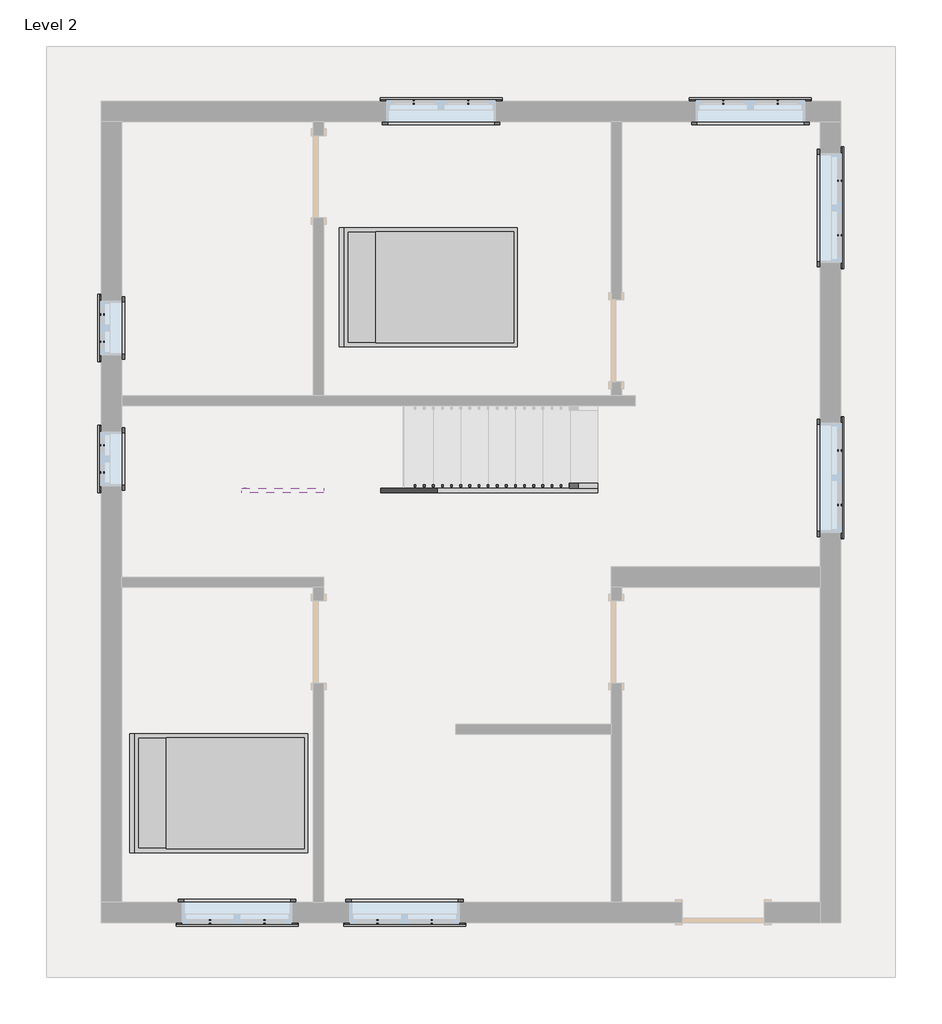
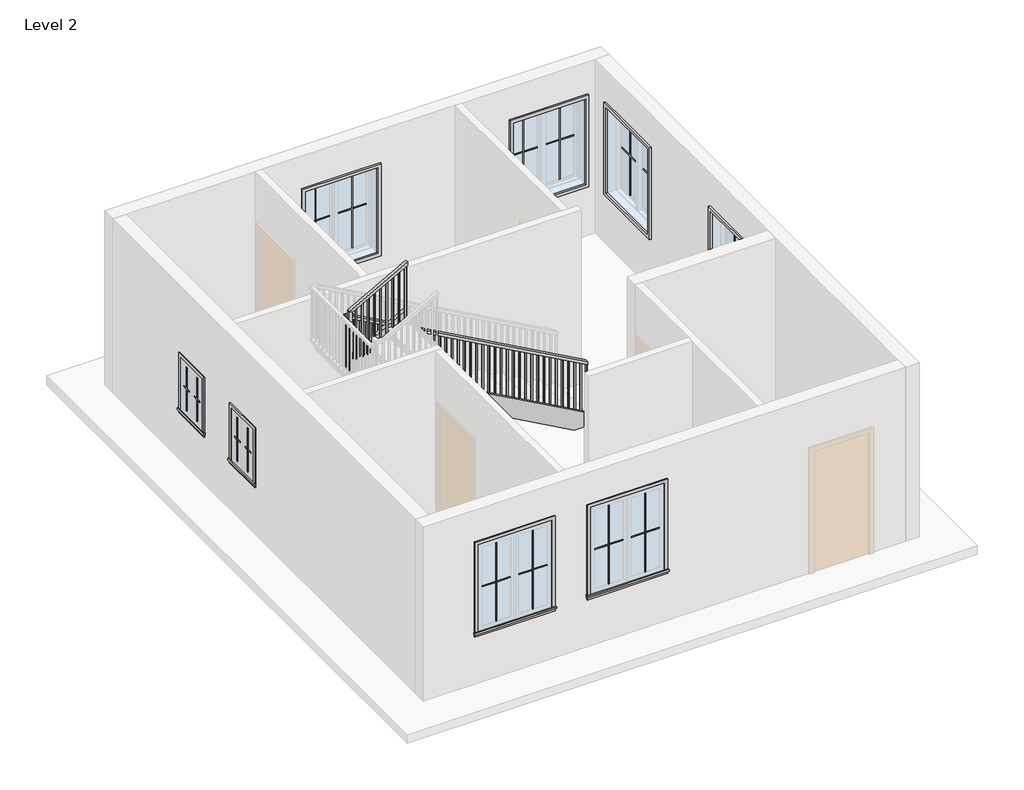
# One storey, part 2 of 2: 32 proxies, 3 members, 2 furniture elements, 1 railing.
"""IFC4 building model written with IfcOpenShell, lengths in millimetres."""

from ifc_helpers import new_model, si_unit, frame, origin, place, context, project, spatial, polyline, outline, extrude, faceted_brep, transform, mapped, element, save
from components import muntin_pattern_2x2_muntin_pattern_2x2_53152e2c, muntin_pattern_2x2_muntin_pattern_2x2_e8f3e573, muntin_pattern_2x2_muntin_pattern_2x2_6dad3731, muntin_pattern_2x2_muntin_pattern_2x2_a30a3345, trim_window_exterior_flat_with_sill_a665a915, trim_window_exterior_flat_with_sill_92b9b949, trim_window_interior_flat_picture_frame_d485c387, trim_window_interior_flat_picture_frame_3bb882cf, bed_17739_bed_17739_15c61121

model = new_model("IFC4")

# Units and contexts
model_context = context("Model", 3, world=origin())
ifc_project = project(units=[si_unit("LENGTHUNIT", "METRE", prefix="MILLI")], contexts=[model_context])

# Site, building, storey
site = spatial("IfcSite", under=ifc_project)
building = spatial("IfcBuilding", under=site)
storey = spatial("IfcBuildingStorey", under=building, Name="Level 2", Elevation=3048.0)

# Proxies
placement = place(None, origin())
muntin_pattern_2x2_muntin_pattern_2x2_shape = muntin_pattern_2x2_muntin_pattern_2x2_53152e2c(model_context)
element("IfcBuildingElementProxy", 1, Name="Muntin Pattern_2x2 : Muntin Pattern_2x2", ObjectType="Muntin Pattern_2x2 : Muntin Pattern_2x2", at=placement, inside=storey, context=model_context, shape_type="MappedRepresentation", body=[
    mapped(muntin_pattern_2x2_muntin_pattern_2x2_shape, transform((1279.525, 12101.9997886, 4032.25), x_axis=(0.0, 1.0, 0.0), y_axis=(-1.0, 0.0, 0.0), z_axis=(0.0, 0.0, 1.0))),
])
element("IfcBuildingElementProxy", 2, Name="Muntin Pattern_2x2 : Muntin Pattern_2x2", ObjectType="Muntin Pattern_2x2 : Muntin Pattern_2x2", at=placement, inside=storey, context=model_context, shape_type="MappedRepresentation", body=[
    mapped(muntin_pattern_2x2_muntin_pattern_2x2_shape, transform((1279.525, 10644.6747886, 4032.25), x_axis=(0.0, 1.0, 0.0), y_axis=(-1.0, 0.0, 0.0), z_axis=(0.0, 0.0, 1.0))),
])
muntin_pattern_2x2_muntin_pattern_2x2_2_shape = muntin_pattern_2x2_muntin_pattern_2x2_e8f3e573(model_context)
element("IfcBuildingElementProxy", 3, Name="Muntin Pattern_2x2 : Muntin Pattern_2x2", ObjectType="Muntin Pattern_2x2 : Muntin Pattern_2x2", at=placement, inside=storey, context=model_context, shape_type="MappedRepresentation", body=[
    mapped(muntin_pattern_2x2_muntin_pattern_2x2_2_shape, transform((1279.525, 12403.6247886, 4032.25), x_axis=(0.0, -1.0, 0.0), y_axis=(1.0, 0.0, 0.0), z_axis=(0.0, 0.0, 1.0))),
])
element("IfcBuildingElementProxy", 4, Name="Muntin Pattern_2x2 : Muntin Pattern_2x2", ObjectType="Muntin Pattern_2x2 : Muntin Pattern_2x2", at=placement, inside=storey, context=model_context, shape_type="MappedRepresentation", body=[
    mapped(muntin_pattern_2x2_muntin_pattern_2x2_2_shape, transform((1279.525, 10946.2997886, 4032.25), x_axis=(0.0, -1.0, 0.0), y_axis=(1.0, 0.0, 0.0), z_axis=(0.0, 0.0, 1.0))),
])
muntin_pattern_2x2_muntin_pattern_2x2_3_shape = muntin_pattern_2x2_muntin_pattern_2x2_6dad3731(model_context)
element("IfcBuildingElementProxy", 5, Name="Muntin Pattern_2x2 : Muntin Pattern_2x2", ObjectType="Muntin Pattern_2x2 : Muntin Pattern_2x2", at=placement, inside=storey, context=model_context, shape_type="MappedRepresentation", body=[
    mapped(muntin_pattern_2x2_muntin_pattern_2x2_3_shape, transform((9490.075, 13892.6997886, 4032.25), x_axis=(0.0, -1.0, 0.0), y_axis=(1.0, 0.0, 0.0), z_axis=(0.0, 0.0, 1.0))),
])
element("IfcBuildingElementProxy", 6, Name="Muntin Pattern_2x2 : Muntin Pattern_2x2", ObjectType="Muntin Pattern_2x2 : Muntin Pattern_2x2", at=placement, inside=storey, context=model_context, shape_type="MappedRepresentation", body=[
    mapped(muntin_pattern_2x2_muntin_pattern_2x2_3_shape, transform((8193.0875, 14767.4122886, 4032.25), x_axis=(1.0, 0.0, 0.0), y_axis=(0.0, 1.0, 0.0), z_axis=(0.0, 0.0, 1.0))),
])
element("IfcBuildingElementProxy", 7, Name="Muntin Pattern_2x2 : Muntin Pattern_2x2", ObjectType="Muntin Pattern_2x2 : Muntin Pattern_2x2", at=placement, inside=storey, context=model_context, shape_type="MappedRepresentation", body=[
    mapped(muntin_pattern_2x2_muntin_pattern_2x2_3_shape, transform((4749.8, 14767.4122886, 4032.25), x_axis=(1.0, 0.0, 0.0), y_axis=(0.0, 1.0, 0.0), z_axis=(0.0, 0.0, 1.0))),
])
element("IfcBuildingElementProxy", 8, Name="Muntin Pattern_2x2 : Muntin Pattern_2x2", ObjectType="Muntin Pattern_2x2 : Muntin Pattern_2x2", at=placement, inside=storey, context=model_context, shape_type="MappedRepresentation", body=[
    mapped(muntin_pattern_2x2_muntin_pattern_2x2_3_shape, transform((9490.075, 10889.1497886, 4032.25), x_axis=(0.0, -1.0, 0.0), y_axis=(1.0, 0.0, 0.0), z_axis=(0.0, 0.0, 1.0))),
])
element("IfcBuildingElementProxy", 9, Name="Muntin Pattern_2x2 : Muntin Pattern_2x2", ObjectType="Muntin Pattern_2x2 : Muntin Pattern_2x2", at=placement, inside=storey, context=model_context, shape_type="MappedRepresentation", body=[
    mapped(muntin_pattern_2x2_muntin_pattern_2x2_3_shape, transform((4950.6207347, 5642.4622886, 4032.25), x_axis=(-1.0, 0.0, 0.0), y_axis=(0.0, -1.0, 0.0), z_axis=(0.0, 0.0, 1.0))),
])
element("IfcBuildingElementProxy", 10, Name="Muntin Pattern_2x2 : Muntin Pattern_2x2", ObjectType="Muntin Pattern_2x2 : Muntin Pattern_2x2", at=placement, inside=storey, context=model_context, shape_type="MappedRepresentation", body=[
    mapped(muntin_pattern_2x2_muntin_pattern_2x2_3_shape, transform((3086.1019847, 5642.4622886, 4032.25), x_axis=(-1.0, 0.0, 0.0), y_axis=(0.0, -1.0, 0.0), z_axis=(0.0, 0.0, 1.0))),
])
muntin_pattern_2x2_muntin_pattern_2x2_4_shape = muntin_pattern_2x2_muntin_pattern_2x2_a30a3345(model_context)
element("IfcBuildingElementProxy", 11, Name="Muntin Pattern_2x2 : Muntin Pattern_2x2", ObjectType="Muntin Pattern_2x2 : Muntin Pattern_2x2", at=placement, inside=storey, context=model_context, shape_type="MappedRepresentation", body=[
    mapped(muntin_pattern_2x2_muntin_pattern_2x2_4_shape, transform((9490.075, 13286.2747886, 4032.25), x_axis=(0.0, 1.0, 0.0), y_axis=(-1.0, 0.0, 0.0), z_axis=(0.0, 0.0, 1.0))),
])
element("IfcBuildingElementProxy", 12, Name="Muntin Pattern_2x2 : Muntin Pattern_2x2", ObjectType="Muntin Pattern_2x2 : Muntin Pattern_2x2", at=placement, inside=storey, context=model_context, shape_type="MappedRepresentation", body=[
    mapped(muntin_pattern_2x2_muntin_pattern_2x2_4_shape, transform((8799.5125, 14767.4122886, 4032.25), x_axis=(-1.0, 0.0, 0.0), y_axis=(0.0, -1.0, 0.0), z_axis=(0.0, 0.0, 1.0))),
])
element("IfcBuildingElementProxy", 13, Name="Muntin Pattern_2x2 : Muntin Pattern_2x2", ObjectType="Muntin Pattern_2x2 : Muntin Pattern_2x2", at=placement, inside=storey, context=model_context, shape_type="MappedRepresentation", body=[
    mapped(muntin_pattern_2x2_muntin_pattern_2x2_4_shape, transform((5356.225, 14767.4122886, 4032.25), x_axis=(-1.0, 0.0, 0.0), y_axis=(0.0, -1.0, 0.0), z_axis=(0.0, 0.0, 1.0))),
])
element("IfcBuildingElementProxy", 14, Name="Muntin Pattern_2x2 : Muntin Pattern_2x2", ObjectType="Muntin Pattern_2x2 : Muntin Pattern_2x2", at=placement, inside=storey, context=model_context, shape_type="MappedRepresentation", body=[
    mapped(muntin_pattern_2x2_muntin_pattern_2x2_4_shape, transform((9490.075, 10282.7247886, 4032.25), x_axis=(0.0, 1.0, 0.0), y_axis=(-1.0, 0.0, 0.0), z_axis=(0.0, 0.0, 1.0))),
])
element("IfcBuildingElementProxy", 15, Name="Muntin Pattern_2x2 : Muntin Pattern_2x2", ObjectType="Muntin Pattern_2x2 : Muntin Pattern_2x2", at=placement, inside=storey, context=model_context, shape_type="MappedRepresentation", body=[
    mapped(muntin_pattern_2x2_muntin_pattern_2x2_4_shape, transform((4344.1957347, 5642.4622886, 4032.25), x_axis=(1.0, 0.0, 0.0), y_axis=(0.0, 1.0, 0.0), z_axis=(0.0, 0.0, 1.0))),
])
element("IfcBuildingElementProxy", 16, Name="Muntin Pattern_2x2 : Muntin Pattern_2x2", ObjectType="Muntin Pattern_2x2 : Muntin Pattern_2x2", at=placement, inside=storey, context=model_context, shape_type="MappedRepresentation", body=[
    mapped(muntin_pattern_2x2_muntin_pattern_2x2_4_shape, transform((2479.6769847, 5642.4622886, 4032.25), x_axis=(1.0, 0.0, 0.0), y_axis=(0.0, 1.0, 0.0), z_axis=(0.0, 0.0, 1.0))),
])
trim_window_exterior_flat_with_sill_shape = trim_window_exterior_flat_with_sill_a665a915(model_context)
element("IfcBuildingElementProxy", 17, Name="Trim-Window-Exterior-Flat : with Sill", ObjectType="Trim-Window-Exterior-Flat : with Sill", at=placement, inside=storey, context=model_context, shape_type="MappedRepresentation", body=[
    mapped(trim_window_exterior_flat_with_sill_shape, transform((1270.0, 12252.8122886, 4876.8), x_axis=(0.0, -1.0, 0.0), y_axis=(0.0, 0.0, 1.0), z_axis=(-1.0, 0.0, 0.0))),
])
element("IfcBuildingElementProxy", 18, Name="Trim-Window-Exterior-Flat : with Sill", ObjectType="Trim-Window-Exterior-Flat : with Sill", at=placement, inside=storey, context=model_context, shape_type="MappedRepresentation", body=[
    mapped(trim_window_exterior_flat_with_sill_shape, transform((1270.0, 10795.4872886, 4876.8), x_axis=(0.0, -1.0, 0.0), y_axis=(0.0, 0.0, 1.0), z_axis=(-1.0, 0.0, 0.0))),
])
trim_window_exterior_flat_with_sill_2_shape = trim_window_exterior_flat_with_sill_92b9b949(model_context)
element("IfcBuildingElementProxy", 19, Name="Trim-Window-Exterior-Flat : with Sill", ObjectType="Trim-Window-Exterior-Flat : with Sill", at=placement, inside=storey, context=model_context, shape_type="MappedRepresentation", body=[
    mapped(trim_window_exterior_flat_with_sill_2_shape, transform((9499.6, 13589.4872886, 5486.4), x_axis=(0.0, 1.0, 0.0), y_axis=(0.0, 0.0, 1.0), z_axis=(1.0, 0.0, 0.0))),
])
element("IfcBuildingElementProxy", 20, Name="Trim-Window-Exterior-Flat : with Sill", ObjectType="Trim-Window-Exterior-Flat : with Sill", at=placement, inside=storey, context=model_context, shape_type="MappedRepresentation", body=[
    mapped(trim_window_exterior_flat_with_sill_2_shape, transform((8496.3, 14776.9372886, 5486.4), x_axis=(-1.0, 0.0, 0.0), y_axis=(0.0, 0.0, 1.0), z_axis=(0.0, 1.0, 0.0))),
])
element("IfcBuildingElementProxy", 21, Name="Trim-Window-Exterior-Flat : with Sill", ObjectType="Trim-Window-Exterior-Flat : with Sill", at=placement, inside=storey, context=model_context, shape_type="MappedRepresentation", body=[
    mapped(trim_window_exterior_flat_with_sill_2_shape, transform((5053.0125, 14776.9372886, 5486.4), x_axis=(-1.0, 0.0, 0.0), y_axis=(0.0, 0.0, 1.0), z_axis=(0.0, 1.0, 0.0))),
])
element("IfcBuildingElementProxy", 22, Name="Trim-Window-Exterior-Flat : with Sill", ObjectType="Trim-Window-Exterior-Flat : with Sill", at=placement, inside=storey, context=model_context, shape_type="MappedRepresentation", body=[
    mapped(trim_window_exterior_flat_with_sill_2_shape, transform((9499.6, 10585.9372886, 5486.4), x_axis=(0.0, 1.0, 0.0), y_axis=(0.0, 0.0, 1.0), z_axis=(1.0, 0.0, 0.0))),
])
element("IfcBuildingElementProxy", 23, Name="Trim-Window-Exterior-Flat : with Sill", ObjectType="Trim-Window-Exterior-Flat : with Sill", at=placement, inside=storey, context=model_context, shape_type="MappedRepresentation", body=[
    mapped(trim_window_exterior_flat_with_sill_2_shape, transform((4647.4082347, 5632.9372886, 5486.4), x_axis=(1.0, 0.0, 0.0), y_axis=(0.0, 0.0, 1.0), z_axis=(0.0, -1.0, 0.0))),
])
element("IfcBuildingElementProxy", 24, Name="Trim-Window-Exterior-Flat : with Sill", ObjectType="Trim-Window-Exterior-Flat : with Sill", at=placement, inside=storey, context=model_context, shape_type="MappedRepresentation", body=[
    mapped(trim_window_exterior_flat_with_sill_2_shape, transform((2782.8894847, 5632.9372886, 5486.4), x_axis=(1.0, 0.0, 0.0), y_axis=(0.0, 0.0, 1.0), z_axis=(0.0, -1.0, 0.0))),
])
trim_window_interior_flat_picture_frame_shape = trim_window_interior_flat_picture_frame_d485c387(model_context)
element("IfcBuildingElementProxy", 25, Name="Trim-Window-Interior-Flat : Picture Frame", ObjectType="Trim-Window-Interior-Flat : Picture Frame", at=placement, inside=storey, context=model_context, shape_type="MappedRepresentation", body=[
    mapped(trim_window_interior_flat_picture_frame_shape, transform((1498.6, 12252.8122886, 4876.8), x_axis=(0.0, 1.0, 0.0), y_axis=(0.0, 0.0, 1.0), z_axis=(1.0, 0.0, 0.0))),
])
element("IfcBuildingElementProxy", 26, Name="Trim-Window-Interior-Flat : Picture Frame", ObjectType="Trim-Window-Interior-Flat : Picture Frame", at=placement, inside=storey, context=model_context, shape_type="MappedRepresentation", body=[
    mapped(trim_window_interior_flat_picture_frame_shape, transform((1498.6, 10795.4872886, 4876.8), x_axis=(0.0, 1.0, 0.0), y_axis=(0.0, 0.0, 1.0), z_axis=(1.0, 0.0, 0.0))),
])
trim_window_interior_flat_picture_frame_2_shape = trim_window_interior_flat_picture_frame_3bb882cf(model_context)
element("IfcBuildingElementProxy", 27, Name="Trim-Window-Interior-Flat : Picture Frame", ObjectType="Trim-Window-Interior-Flat : Picture Frame", at=placement, inside=storey, context=model_context, shape_type="MappedRepresentation", body=[
    mapped(trim_window_interior_flat_picture_frame_2_shape, transform((9271.0, 13589.4872886, 5486.4), x_axis=(0.0, -1.0, 0.0), y_axis=(0.0, 0.0, 1.0), z_axis=(-1.0, 0.0, 0.0))),
])
element("IfcBuildingElementProxy", 28, Name="Trim-Window-Interior-Flat : Picture Frame", ObjectType="Trim-Window-Interior-Flat : Picture Frame", at=placement, inside=storey, context=model_context, shape_type="MappedRepresentation", body=[
    mapped(trim_window_interior_flat_picture_frame_2_shape, transform((8496.3, 14548.3372886, 5486.4), x_axis=(1.0, 0.0, 0.0), y_axis=(0.0, 0.0, 1.0), z_axis=(0.0, -1.0, 0.0))),
])
element("IfcBuildingElementProxy", 29, Name="Trim-Window-Interior-Flat : Picture Frame", ObjectType="Trim-Window-Interior-Flat : Picture Frame", at=placement, inside=storey, context=model_context, shape_type="MappedRepresentation", body=[
    mapped(trim_window_interior_flat_picture_frame_2_shape, transform((5053.0125, 14548.3372886, 5486.4), x_axis=(1.0, 0.0, 0.0), y_axis=(0.0, 0.0, 1.0), z_axis=(0.0, -1.0, 0.0))),
])
element("IfcBuildingElementProxy", 30, Name="Trim-Window-Interior-Flat : Picture Frame", ObjectType="Trim-Window-Interior-Flat : Picture Frame", at=placement, inside=storey, context=model_context, shape_type="MappedRepresentation", body=[
    mapped(trim_window_interior_flat_picture_frame_2_shape, transform((9271.0, 10585.9372886, 5486.4), x_axis=(0.0, -1.0, 0.0), y_axis=(0.0, 0.0, 1.0), z_axis=(-1.0, 0.0, 0.0))),
])
element("IfcBuildingElementProxy", 31, Name="Trim-Window-Interior-Flat : Picture Frame", ObjectType="Trim-Window-Interior-Flat : Picture Frame", at=placement, inside=storey, context=model_context, shape_type="MappedRepresentation", body=[
    mapped(trim_window_interior_flat_picture_frame_2_shape, transform((4647.4082347, 5861.5372886, 5486.4), x_axis=(-1.0, 0.0, 0.0), y_axis=(0.0, 0.0, 1.0), z_axis=(0.0, 1.0, 0.0))),
])
element("IfcBuildingElementProxy", 32, Name="Trim-Window-Interior-Flat : Picture Frame", ObjectType="Trim-Window-Interior-Flat : Picture Frame", at=placement, inside=storey, context=model_context, shape_type="MappedRepresentation", body=[
    mapped(trim_window_interior_flat_picture_frame_2_shape, transform((2782.8894847, 5861.5372886, 5486.4), x_axis=(-1.0, 0.0, 0.0), y_axis=(0.0, 0.0, 1.0), z_axis=(0.0, 1.0, 0.0))),
])

# Furniture
bed_17739_bed_17739_shape = bed_17739_bed_17739_15c61121(model_context)
element("IfcFurniture", 33, ObjectType="Bed_17739 : Bed_17739", at=placement, inside=storey, context=model_context, shape_type="MappedRepresentation", body=[
    mapped(bed_17739_bed_17739_shape, transform((4933.95, 12706.8372886, 3048.0), x_axis=(0.0, 1.0, 0.0), y_axis=(-1.0, 0.0, 0.0), z_axis=(0.0, 0.0, 1.0))),
])
element("IfcFurniture", 34, ObjectType="Bed_17739 : Bed_17739", at=placement, inside=storey, context=model_context, shape_type="MappedRepresentation", body=[
    mapped(bed_17739_bed_17739_shape, transform((2603.5, 7074.3872886, 3048.0), x_axis=(0.0, 1.0, 0.0), y_axis=(-1.0, 0.0, 0.0), z_axis=(0.0, 0.0, 1.0))),
])

# Members
element("IfcMember", 35, ObjectType="Stringer - 2\" Width", at=placement, inside=storey, context=model_context, shape_type="SweptSolid", body=[
    extrude(outline(polyline([(3048.0, 6794.5), (3255.5983948, 6794.5), (5428.7095059, 2882.9), (5080.0308318, 2882.9), (3048.0, 6540.5554972), (3048.0, 6794.5)])), frame((0.0, 10420.8372886, 0.0), z_axis=(0.0, 1.0, 0.0), x_axis=(0.0, 0.0, 1.0)), (0.0, 0.0, 1.0), 50.8),
])
element("IfcMember", 36, ObjectType="Stringer - 2\" Width", at=placement, inside=storey, context=model_context, shape_type="SweptSolid", body=[
    extrude(outline(polyline([(2832.1, 10471.6372886), (2882.9, 10471.6372886), (2882.9, 10469.0972886), (2832.1, 10469.0972886), (2832.1, 10471.6372886)])), frame((0.0, 0.0, 5190.0666667), z_axis=(0.0, 0.0, 1.0), x_axis=(1.0, 0.0, 0.0)), (0.0, 0.0, 1.0), 304.8),
])
element("IfcMember", 37, ObjectType="Stringer - 2\" Width", at=placement, inside=storey, context=model_context, shape_type="SweptSolid", body=[
    extrude(outline(polyline([(5626.2650614, 2832.1), (5277.5863873, 2832.1), (5785.5874899, 3746.5019847), (6134.266164, 3746.5019847), (5626.2650614, 2832.1)])), frame((0.0, 10418.2972886, 0.0), z_axis=(0.0, 1.0, 0.0), x_axis=(0.0, 0.0, 1.0)), (0.0, 0.0, 1.0), 50.8),
])

# Railing
element("IfcRailing", 38, ObjectType="Handrail - Rectangular", at=placement, inside=storey, context=model_context, shape_type="SolidModel", body=[
    faceted_brep([(6794.5, 10471.6372886, 4131.7333333), (6794.5, 10471.6372886, 4073.620221), (6794.5, 10522.4372886, 4073.620221), (6794.5, 10522.4372886, 4131.7333333), (2908.3, 10471.6372886, 6290.7333333), (2857.5, 10471.6372886, 6260.8424432), (2857.5, 10522.4372886, 6260.8424432), (2908.3, 10522.4372886, 6290.7333333), (2908.3, 10471.6372886, 6333.0666667), (2857.5, 10471.6372886, 6282.2666667), (2857.5, 10522.4372886, 6282.2666667), (2908.3, 10522.4372886, 6333.0666667), (2832.1, 10471.6372886, 6333.0666667), (2832.1, 10471.6372886, 6282.2666667), (2781.3, 10522.4372886, 6282.2666667), (2781.3, 10522.4372886, 6333.0666667), (2832.1, 10395.4372886, 6333.0666667), (2832.1, 10395.4372886, 6282.2666667), (2781.3, 10395.4372886, 6282.2666667), (2781.3, 10395.4372886, 6333.0666667), (2832.1, 10392.8972886, 6333.0666667), (2781.3, 10392.8972886, 6333.0666667), (2781.3, 10392.8972886, 6282.2666667), (2832.1, 10392.8972886, 6282.2666667)], [[[0, 1, 2, 3]], [[1, 0, 4, 5]], [[2, 1, 5, 6]], [[3, 2, 6, 7]], [[0, 3, 7, 4]], [[5, 4, 8, 9]], [[6, 5, 9, 10]], [[7, 6, 10, 11]], [[4, 7, 11, 8]], [[9, 8, 12, 13]], [[10, 9, 13, 14]], [[11, 10, 14, 15]], [[8, 11, 15, 12]], [[13, 12, 16, 17]], [[14, 13, 17, 18]], [[15, 14, 18, 19]], [[12, 15, 19, 16]], [[20, 21, 22, 23]], [[17, 16, 20, 23]], [[18, 17, 23, 22]], [[19, 18, 22, 21]], [[16, 19, 21, 20]]]),
    faceted_brep([(2832.1, 10418.2972886, 6333.0666667), (2832.1, 10367.4972886, 6282.2666667), (2781.3, 10367.4972886, 6282.2666667), (2781.3, 10418.2972886, 6333.0666667), (2832.1, 10418.2972886, 6444.2869174), (2781.3, 10418.2972886, 6474.177839), (2781.3, 10367.4972886, 6474.177839), (2832.1, 10367.4972886, 6444.2869174)], [[[0, 1, 2, 3]], [[4, 5, 6, 7]], [[1, 0, 4, 7]], [[2, 1, 7, 6]], [[3, 2, 6, 5]], [[0, 3, 5, 4]]]),
    faceted_brep([(2781.3, 10418.2972886, 6474.177839), (2832.1, 10418.2972886, 6444.2869174), (2832.1, 10367.4972886, 6444.2869174), (2781.3, 10367.4972886, 6474.177839), (3746.5019847, 10418.2972886, 7010.4), (3746.5019847, 10367.4972886, 7010.4), (3746.5019847, 10367.4972886, 6952.2869174), (3746.5019847, 10418.2972886, 6952.2869174)], [[[0, 1, 2, 3]], [[4, 5, 6, 7]], [[1, 0, 4, 7]], [[2, 1, 7, 6]], [[3, 2, 6, 5]], [[0, 3, 5, 4]]]),
    extrude(outline(polyline([(6932.8838142, 3711.575), (5926.6666667, 3711.575), (5926.6666667, 3730.625), (6943.4671246, 3730.625), (6932.8838142, 3711.575)])), frame((0.0, 10383.3722886, 0.0), z_axis=(0.0, 1.0, 0.0), x_axis=(0.0, 0.0, 1.0)), (0.0, 0.0, 1.0), 19.05),
    extrude(outline(polyline([(6876.4394923, 3609.975), (5926.6666667, 3609.975), (5926.6666667, 3629.025), (6887.0228026, 3629.025), (6876.4394923, 3609.975)])), frame((0.0, 10383.3722886, 0.0), z_axis=(0.0, 1.0, 0.0), x_axis=(0.0, 0.0, 1.0)), (0.0, 0.0, 1.0), 19.05),
    extrude(outline(polyline([(6819.9951703, 3508.375), (5926.6666667, 3508.375), (5926.6666667, 3527.425), (6830.5784807, 3527.425), (6819.9951703, 3508.375)])), frame((0.0, 10383.3722886, 0.0), z_axis=(0.0, 1.0, 0.0), x_axis=(0.0, 0.0, 1.0)), (0.0, 0.0, 1.0), 19.05),
    extrude(outline(polyline([(6763.5504809, 3406.775), (5757.3333333, 3406.775), (5757.3333333, 3425.825), (6774.1337912, 3425.825), (6763.5504809, 3406.775)])), frame((0.0, 10383.3722886, 0.0), z_axis=(0.0, 1.0, 0.0), x_axis=(0.0, 0.0, 1.0)), (0.0, 0.0, 1.0), 19.05),
    extrude(outline(polyline([(6707.1061589, 3305.175), (5757.3333333, 3305.175), (5757.3333333, 3324.225), (6717.6894693, 3324.225), (6707.1061589, 3305.175)])), frame((0.0, 10383.3722886, 0.0), z_axis=(0.0, 1.0, 0.0), x_axis=(0.0, 0.0, 1.0)), (0.0, 0.0, 1.0), 19.05),
    extrude(outline(polyline([(6650.661837, 3203.575), (5757.3333333, 3203.575), (5757.3333333, 3222.625), (6661.2451474, 3222.625), (6650.661837, 3203.575)])), frame((0.0, 10383.3722886, 0.0), z_axis=(0.0, 1.0, 0.0), x_axis=(0.0, 0.0, 1.0)), (0.0, 0.0, 1.0), 19.05),
    extrude(outline(polyline([(6594.2171475, 3101.975), (5588.0, 3101.975), (5588.0, 3121.025), (6604.8004579, 3121.025), (6594.2171475, 3101.975)])), frame((0.0, 10383.3722886, 0.0), z_axis=(0.0, 1.0, 0.0), x_axis=(0.0, 0.0, 1.0)), (0.0, 0.0, 1.0), 19.05),
    extrude(outline(polyline([(6537.7728256, 3000.375), (5588.0, 3000.375), (5588.0, 3019.425), (6548.356136, 3019.425), (6537.7728256, 3000.375)])), frame((0.0, 10383.3722886, 0.0), z_axis=(0.0, 1.0, 0.0), x_axis=(0.0, 0.0, 1.0)), (0.0, 0.0, 1.0), 19.05),
    extrude(outline(polyline([(6481.3285037, 2898.775), (5588.0, 2898.775), (5588.0, 2917.825), (6491.911814, 2917.825), (6481.3285037, 2898.775)])), frame((0.0, 10383.3722886, 0.0), z_axis=(0.0, 1.0, 0.0), x_axis=(0.0, 0.0, 1.0)), (0.0, 0.0, 1.0), 19.05),
    extrude(outline(polyline([(2816.225, 10404.9622886), (2816.225, 10385.9122886), (2797.175, 10385.9122886), (2797.175, 10404.9622886), (2816.225, 10404.9622886)])), frame((0.0, 0.0, 5418.6666667), z_axis=(0.0, 0.0, 1.0), x_axis=(1.0, 0.0, 0.0)), (0.0, 0.0, 1.0), 863.6),
    extrude(outline(polyline([(2841.625, 10487.5122886), (2822.575, 10487.5122886), (2822.575, 10506.5622886), (2841.625, 10506.5622886), (2841.625, 10487.5122886)])), frame((0.0, 0.0, 5418.6666667), z_axis=(0.0, 0.0, 1.0), x_axis=(1.0, 0.0, 0.0)), (0.0, 0.0, 1.0), 863.6),
    extrude(outline(polyline([(6223.8007765, 2924.175), (5249.3333333, 2924.175), (5249.3333333, 2943.225), (6213.2174432, 2943.225), (6223.8007765, 2924.175)])), frame((0.0, 10487.5122886, 0.0), z_axis=(0.0, 1.0, 0.0), x_axis=(0.0, 0.0, 1.0)), (0.0, 0.0, 1.0), 19.05),
    extrude(outline(polyline([(6167.3563321, 3025.775), (5249.3333333, 3025.775), (5249.3333333, 3044.825), (6156.7729988, 3044.825), (6167.3563321, 3025.775)])), frame((0.0, 10487.5122886, 0.0), z_axis=(0.0, 1.0, 0.0), x_axis=(0.0, 0.0, 1.0)), (0.0, 0.0, 1.0), 19.05),
    extrude(outline(polyline([(6110.9118876, 3127.375), (5249.3333333, 3127.375), (5249.3333333, 3146.425), (6100.3285543, 3146.425), (6110.9118876, 3127.375)])), frame((0.0, 10487.5122886, 0.0), z_axis=(0.0, 1.0, 0.0), x_axis=(0.0, 0.0, 1.0)), (0.0, 0.0, 1.0), 19.05),
    extrude(outline(polyline([(6054.4674432, 3228.975), (5080.0, 3228.975), (5080.0, 3248.025), (6043.8841099, 3248.025), (6054.4674432, 3228.975)])), frame((0.0, 10487.5122886, 0.0), z_axis=(0.0, 1.0, 0.0), x_axis=(0.0, 0.0, 1.0)), (0.0, 0.0, 1.0), 19.05),
    extrude(outline(polyline([(5998.0229988, 3330.575), (5080.0, 3330.575), (5080.0, 3349.625), (5987.4396654, 3349.625), (5998.0229988, 3330.575)])), frame((0.0, 10487.5122886, 0.0), z_axis=(0.0, 1.0, 0.0), x_axis=(0.0, 0.0, 1.0)), (0.0, 0.0, 1.0), 19.05),
    extrude(outline(polyline([(5941.5785543, 3432.175), (5080.0, 3432.175), (5080.0, 3451.225), (5930.995221, 3451.225), (5941.5785543, 3432.175)])), frame((0.0, 10487.5122886, 0.0), z_axis=(0.0, 1.0, 0.0), x_axis=(0.0, 0.0, 1.0)), (0.0, 0.0, 1.0), 19.05),
    extrude(outline(polyline([(5885.1341099, 3533.775), (4910.6666667, 3533.775), (4910.6666667, 3552.825), (5874.5507765, 3552.825), (5885.1341099, 3533.775)])), frame((0.0, 10487.5122886, 0.0), z_axis=(0.0, 1.0, 0.0), x_axis=(0.0, 0.0, 1.0)), (0.0, 0.0, 1.0), 19.05),
    extrude(outline(polyline([(5828.6896654, 3635.375), (4910.6666667, 3635.375), (4910.6666667, 3654.425), (5818.1063321, 3654.425), (5828.6896654, 3635.375)])), frame((0.0, 10487.5122886, 0.0), z_axis=(0.0, 1.0, 0.0), x_axis=(0.0, 0.0, 1.0)), (0.0, 0.0, 1.0), 19.05),
    extrude(outline(polyline([(5772.245221, 3736.975), (4910.6666667, 3736.975), (4910.6666667, 3756.025), (5761.6618876, 3756.025), (5772.245221, 3736.975)])), frame((0.0, 10487.5122886, 0.0), z_axis=(0.0, 1.0, 0.0), x_axis=(0.0, 0.0, 1.0)), (0.0, 0.0, 1.0), 19.05),
    extrude(outline(polyline([(5715.8007765, 3838.575), (4741.3333333, 3838.575), (4741.3333333, 3857.625), (5705.2174432, 3857.625), (5715.8007765, 3838.575)])), frame((0.0, 10487.5122886, 0.0), z_axis=(0.0, 1.0, 0.0), x_axis=(0.0, 0.0, 1.0)), (0.0, 0.0, 1.0), 19.05),
    extrude(outline(polyline([(5659.3563321, 3940.175), (4741.3333333, 3940.175), (4741.3333333, 3959.225), (5648.7729988, 3959.225), (5659.3563321, 3940.175)])), frame((0.0, 10487.5122886, 0.0), z_axis=(0.0, 1.0, 0.0), x_axis=(0.0, 0.0, 1.0)), (0.0, 0.0, 1.0), 19.05),
    extrude(outline(polyline([(5602.9118876, 4041.775), (4741.3333333, 4041.775), (4741.3333333, 4060.825), (5592.3285543, 4060.825), (5602.9118876, 4041.775)])), frame((0.0, 10487.5122886, 0.0), z_axis=(0.0, 1.0, 0.0), x_axis=(0.0, 0.0, 1.0)), (0.0, 0.0, 1.0), 19.05),
    extrude(outline(polyline([(5546.4674432, 4143.375), (4572.0, 4143.375), (4572.0, 4162.425), (5535.8841099, 4162.425), (5546.4674432, 4143.375)])), frame((0.0, 10487.5122886, 0.0), z_axis=(0.0, 1.0, 0.0), x_axis=(0.0, 0.0, 1.0)), (0.0, 0.0, 1.0), 19.05),
    extrude(outline(polyline([(5490.0229988, 4244.975), (4572.0, 4244.975), (4572.0, 4264.025), (5479.4396654, 4264.025), (5490.0229988, 4244.975)])), frame((0.0, 10487.5122886, 0.0), z_axis=(0.0, 1.0, 0.0), x_axis=(0.0, 0.0, 1.0)), (0.0, 0.0, 1.0), 19.05),
    extrude(outline(polyline([(5433.5785543, 4346.575), (4572.0, 4346.575), (4572.0, 4365.625), (5422.995221, 4365.625), (5433.5785543, 4346.575)])), frame((0.0, 10487.5122886, 0.0), z_axis=(0.0, 1.0, 0.0), x_axis=(0.0, 0.0, 1.0)), (0.0, 0.0, 1.0), 19.05),
    extrude(outline(polyline([(5377.1341099, 4448.175), (4402.6666667, 4448.175), (4402.6666667, 4467.225), (5366.5507765, 4467.225), (5377.1341099, 4448.175)])), frame((0.0, 10487.5122886, 0.0), z_axis=(0.0, 1.0, 0.0), x_axis=(0.0, 0.0, 1.0)), (0.0, 0.0, 1.0), 19.05),
    extrude(outline(polyline([(5320.6896654, 4549.775), (4402.6666667, 4549.775), (4402.6666667, 4568.825), (5310.1063321, 4568.825), (5320.6896654, 4549.775)])), frame((0.0, 10487.5122886, 0.0), z_axis=(0.0, 1.0, 0.0), x_axis=(0.0, 0.0, 1.0)), (0.0, 0.0, 1.0), 19.05),
    extrude(outline(polyline([(5264.245221, 4651.375), (4402.6666667, 4651.375), (4402.6666667, 4670.425), (5253.6618876, 4670.425), (5264.245221, 4651.375)])), frame((0.0, 10487.5122886, 0.0), z_axis=(0.0, 1.0, 0.0), x_axis=(0.0, 0.0, 1.0)), (0.0, 0.0, 1.0), 19.05),
    extrude(outline(polyline([(5207.8007765, 4752.975), (4233.3333333, 4752.975), (4233.3333333, 4772.025), (5197.2174432, 4772.025), (5207.8007765, 4752.975)])), frame((0.0, 10487.5122886, 0.0), z_axis=(0.0, 1.0, 0.0), x_axis=(0.0, 0.0, 1.0)), (0.0, 0.0, 1.0), 19.05),
    extrude(outline(polyline([(5151.3563321, 4854.575), (4233.3333333, 4854.575), (4233.3333333, 4873.625), (5140.7729988, 4873.625), (5151.3563321, 4854.575)])), frame((0.0, 10487.5122886, 0.0), z_axis=(0.0, 1.0, 0.0), x_axis=(0.0, 0.0, 1.0)), (0.0, 0.0, 1.0), 19.05),
    extrude(outline(polyline([(5094.9118876, 4956.175), (4233.3333333, 4956.175), (4233.3333333, 4975.225), (5084.3285543, 4975.225), (5094.9118876, 4956.175)])), frame((0.0, 10487.5122886, 0.0), z_axis=(0.0, 1.0, 0.0), x_axis=(0.0, 0.0, 1.0)), (0.0, 0.0, 1.0), 19.05),
    extrude(outline(polyline([(5038.4674432, 5057.775), (4064.0, 5057.775), (4064.0, 5076.825), (5027.8841099, 5076.825), (5038.4674432, 5057.775)])), frame((0.0, 10487.5122886, 0.0), z_axis=(0.0, 1.0, 0.0), x_axis=(0.0, 0.0, 1.0)), (0.0, 0.0, 1.0), 19.05),
    extrude(outline(polyline([(4982.0229988, 5159.375), (4064.0, 5159.375), (4064.0, 5178.425), (4971.4396654, 5178.425), (4982.0229988, 5159.375)])), frame((0.0, 10487.5122886, 0.0), z_axis=(0.0, 1.0, 0.0), x_axis=(0.0, 0.0, 1.0)), (0.0, 0.0, 1.0), 19.05),
    extrude(outline(polyline([(4925.5785543, 5260.975), (4064.0, 5260.975), (4064.0, 5280.025), (4914.995221, 5280.025), (4925.5785543, 5260.975)])), frame((0.0, 10487.5122886, 0.0), z_axis=(0.0, 1.0, 0.0), x_axis=(0.0, 0.0, 1.0)), (0.0, 0.0, 1.0), 19.05),
    extrude(outline(polyline([(4869.1341099, 5362.575), (3894.6666667, 5362.575), (3894.6666667, 5381.625), (4858.5507765, 5381.625), (4869.1341099, 5362.575)])), frame((0.0, 10487.5122886, 0.0), z_axis=(0.0, 1.0, 0.0), x_axis=(0.0, 0.0, 1.0)), (0.0, 0.0, 1.0), 19.05),
    extrude(outline(polyline([(4812.6896654, 5464.175), (3894.6666667, 5464.175), (3894.6666667, 5483.225), (4802.1063321, 5483.225), (4812.6896654, 5464.175)])), frame((0.0, 10487.5122886, 0.0), z_axis=(0.0, 1.0, 0.0), x_axis=(0.0, 0.0, 1.0)), (0.0, 0.0, 1.0), 19.05),
    extrude(outline(polyline([(4756.245221, 5565.775), (3894.6666667, 5565.775), (3894.6666667, 5584.825), (4745.6618876, 5584.825), (4756.245221, 5565.775)])), frame((0.0, 10487.5122886, 0.0), z_axis=(0.0, 1.0, 0.0), x_axis=(0.0, 0.0, 1.0)), (0.0, 0.0, 1.0), 19.05),
    extrude(outline(polyline([(4699.8007765, 5667.375), (3725.3333333, 5667.375), (3725.3333333, 5686.425), (4689.2174432, 5686.425), (4699.8007765, 5667.375)])), frame((0.0, 10487.5122886, 0.0), z_axis=(0.0, 1.0, 0.0), x_axis=(0.0, 0.0, 1.0)), (0.0, 0.0, 1.0), 19.05),
    extrude(outline(polyline([(4643.3563321, 5768.975), (3725.3333333, 5768.975), (3725.3333333, 5788.025), (4632.7729988, 5788.025), (4643.3563321, 5768.975)])), frame((0.0, 10487.5122886, 0.0), z_axis=(0.0, 1.0, 0.0), x_axis=(0.0, 0.0, 1.0)), (0.0, 0.0, 1.0), 19.05),
    extrude(outline(polyline([(4586.9118876, 5870.575), (3725.3333333, 5870.575), (3725.3333333, 5889.625), (4576.3285543, 5889.625), (4586.9118876, 5870.575)])), frame((0.0, 10487.5122886, 0.0), z_axis=(0.0, 1.0, 0.0), x_axis=(0.0, 0.0, 1.0)), (0.0, 0.0, 1.0), 19.05),
    extrude(outline(polyline([(4530.4674432, 5972.175), (3556.0, 5972.175), (3556.0, 5991.225), (4519.8841099, 5991.225), (4530.4674432, 5972.175)])), frame((0.0, 10487.5122886, 0.0), z_axis=(0.0, 1.0, 0.0), x_axis=(0.0, 0.0, 1.0)), (0.0, 0.0, 1.0), 19.05),
    extrude(outline(polyline([(4474.0229988, 6073.775), (3556.0, 6073.775), (3556.0, 6092.825), (4463.4396654, 6092.825), (4474.0229988, 6073.775)])), frame((0.0, 10487.5122886, 0.0), z_axis=(0.0, 1.0, 0.0), x_axis=(0.0, 0.0, 1.0)), (0.0, 0.0, 1.0), 19.05),
    extrude(outline(polyline([(4417.5785543, 6175.375), (3556.0, 6175.375), (3556.0, 6194.425), (4406.995221, 6194.425), (4417.5785543, 6175.375)])), frame((0.0, 10487.5122886, 0.0), z_axis=(0.0, 1.0, 0.0), x_axis=(0.0, 0.0, 1.0)), (0.0, 0.0, 1.0), 19.05),
    extrude(outline(polyline([(4361.1341099, 6276.975), (3386.6666667, 6276.975), (3386.6666667, 6296.025), (4350.5507765, 6296.025), (4361.1341099, 6276.975)])), frame((0.0, 10487.5122886, 0.0), z_axis=(0.0, 1.0, 0.0), x_axis=(0.0, 0.0, 1.0)), (0.0, 0.0, 1.0), 19.05),
    extrude(outline(polyline([(4304.6896654, 6378.575), (3386.6666667, 6378.575), (3386.6666667, 6397.625), (4294.1063321, 6397.625), (4304.6896654, 6378.575)])), frame((0.0, 10487.5122886, 0.0), z_axis=(0.0, 1.0, 0.0), x_axis=(0.0, 0.0, 1.0)), (0.0, 0.0, 1.0), 19.05),
    extrude(outline(polyline([(4248.245221, 6480.175), (3386.6666667, 6480.175), (3386.6666667, 6499.225), (4237.6618876, 6499.225), (4248.245221, 6480.175)])), frame((0.0, 10487.5122886, 0.0), z_axis=(0.0, 1.0, 0.0), x_axis=(0.0, 0.0, 1.0)), (0.0, 0.0, 1.0), 19.05),
    extrude(outline(polyline([(4191.8007765, 6581.775), (3217.3333333, 6581.775), (3217.3333333, 6600.825), (4181.2174432, 6600.825), (4191.8007765, 6581.775)])), frame((0.0, 10487.5122886, 0.0), z_axis=(0.0, 1.0, 0.0), x_axis=(0.0, 0.0, 1.0)), (0.0, 0.0, 1.0), 19.05),
    extrude(outline(polyline([(4135.3563321, 6683.375), (3217.3333333, 6683.375), (3217.3333333, 6702.425), (4124.7729988, 6702.425), (4135.3563321, 6683.375)])), frame((0.0, 10487.5122886, 0.0), z_axis=(0.0, 1.0, 0.0), x_axis=(0.0, 0.0, 1.0)), (0.0, 0.0, 1.0), 19.05),
    extrude(outline(polyline([(2816.225, 10402.4222886), (2816.225, 10383.3722886), (2797.175, 10383.3722886), (2797.175, 10402.4222886), (2816.225, 10402.4222886)])), frame((0.0, 0.0, 5418.6666667), z_axis=(0.0, 0.0, 1.0), x_axis=(1.0, 0.0, 0.0)), (0.0, 0.0, 1.0), 863.6),
    extrude(outline(polyline([(2816.225, 10487.5122886), (2797.175, 10487.5122886), (2797.175, 10506.5622886), (2816.225, 10506.5622886), (2816.225, 10487.5122886)])), frame((0.0, 0.0, 5418.6666667), z_axis=(0.0, 0.0, 1.0), x_axis=(1.0, 0.0, 0.0)), (0.0, 0.0, 1.0), 863.6),
    extrude(outline(polyline([(6941.703607, 3727.4519847), (5926.6666667, 3727.4519847), (5926.6666667, 3746.5019847), (6952.2869174, 3746.5019847), (6941.703607, 3727.4519847)])), frame((0.0, 10383.3722886, 0.0), z_axis=(0.0, 1.0, 0.0), x_axis=(0.0, 0.0, 1.0)), (0.0, 0.0, 1.0), 19.05),
    extrude(outline(polyline([(4084.2035543, 6775.45), (3217.3333333, 6775.45), (3217.3333333, 6794.5), (4073.620221, 6794.5), (4084.2035543, 6775.45)])), frame((0.0, 10487.5122886, 0.0), z_axis=(0.0, 1.0, 0.0), x_axis=(0.0, 0.0, 1.0)), (0.0, 0.0, 1.0), 19.05),
])

save(model, "model.ifc")

# Revit data of these elements
# Type "Muntin Pattern_2x2 : Muntin Pattern_2x2"
#   Width [instance default] = 4' - 0"
#   Thickness = 0' - 0 1/2"
#   Height [instance default] = 4' - 0"
#   Distance = 0' - 0 3/4"
#   Interior Material [instance default] = none
#   Exterior Material [instance default] = none
#   Default Elevation = 0
# Type "Trim-Window-Exterior-Flat : with Sill"
#   Trim Width = 0' - 2 1/4"
#   Trim Thickness_Picture Frame = 0' - 1 1/4"
#   Trim Thickness_with Sill = 0' - 0 3/4"
#   Sill Thickness = 0' - 1 1/4"
#   Opening Width [instance default] = 2' - 0"
#   Opening Height [instance default] = 3' - 0"
#   Default Elevation = 4' - 0"
#   Sill = yes
#   Picture Frame = no
#   Trim Material [instance default] = none
# Type "Trim-Window-Interior-Flat : Picture Frame"
#   Trim Thickness_Picture Frame = 0' - 1 1/4"
#   Trim Width = 0' - 2 1/4"
#   Trim Thickness_with Sill = 0' - 0 3/4"
#   Sill Thickness = 0' - 1 1/4"
#   Opening Width [instance default] = 2' - 0"
#   Opening Height [instance default] = 3' - 0"
#   Default Elevation = 4' - 0"
#   Sill = no
#   Picture Frame = yes
#   Trim Material [instance default] = none
# Type "Bed_17739 : Bed_17739"
#   Default Elevation = 0
# Type "Handrail - Rectangular"
#   Assembly Code = "C2010400"
#   built-in parameter 1008612 = 0.0416667 (stored number, unit not read)
#   built-in parameter 1008611 = 0.0416667 (stored number, unit not read)
#   built-in parameter 1008609 = 0.333333 (stored number, unit not read)
#   built-in parameter 1008604 = 0.166667 (stored number, unit not read)
#   built-in parameter 1008603 = 0.166667 (stored number, unit not read)
#   Railing Height = 3' - 0"
#   built-in parameter 1008630 = 2
#   built-in parameter 1008610 = 2
#   built-in parameter 1008618 = Baluster - Square : 3/4"
# Elements 1, 2, 3, 4 (IfcBuildingElementProxy, "Muntin Pattern_2x2 : Muntin Pattern_2x2")
#   Width = 0' - 6 5/8"
#   Height = 2' - 6 1/2"
#   Interior Material = Wood - Stained
#   Exterior Material = Clad - White
#   Phase Created = New Construction
#   Materials on its faces: "Clad - White", "Wood - Stained"
# Elements 5, 6, 7, 8, 9, 10, 11, 12, 13, 14, 15, 16 (IfcBuildingElementProxy, "Muntin Pattern_2x2 : Muntin Pattern_2x2")
#   Width = 1' - 6 5/8"
#   Height = 4' - 6 1/2"
#   Interior Material = Wood - Stained
#   Exterior Material = Clad - White
#   Phase Created = New Construction
#   Materials on its faces: "Clad - White", "Wood - Stained"
# Elements 17, 18 (IfcBuildingElementProxy, "Trim-Window-Exterior-Flat : with Sill")
#   Opening Width = 2' - 0"
#   Opening Height = 3' - 0"
#   Trim Material = Clad - White
#   Phase Created = New Construction
#   Materials on its faces: "Clad - White"
# Elements 19, 20, 21, 22, 23, 24 (IfcBuildingElementProxy, "Trim-Window-Exterior-Flat : with Sill")
#   Opening Width = 4' - 0"
#   Opening Height = 5' - 0"
#   Trim Material = Clad - White
#   Phase Created = New Construction
#   Materials on its faces: "Clad - White"
# Elements 25, 26 (IfcBuildingElementProxy, "Trim-Window-Interior-Flat : Picture Frame")
#   Opening Width = 2' - 0"
#   Opening Height = 3' - 0"
#   Trim Material = Wood - Stained
#   Phase Created = New Construction
#   Materials on its faces: "Wood - Stained"
# Elements 27, 28, 29, 30, 31, 32 (IfcBuildingElementProxy, "Trim-Window-Interior-Flat : Picture Frame")
#   Opening Width = 4' - 0"
#   Opening Height = 5' - 0"
#   Trim Material = Wood - Stained
#   Phase Created = New Construction
#   Materials on its faces: "Wood - Stained"
# Elements 33, 34 (IfcFurniture, "Bed_17739 : Bed_17739")
#   Phase Created = New Construction
#   Materials on its faces: "legs", "sheets", "bed frame", "Blanket"
# Elements 35, 36, 37 (IfcMember, "Stringer - 2\" Width")
#   Phase Created = New Construction
# Element 38 (IfcRailing, "Handrail - Rectangular")
#   Phase Created = New Construction
# Materials
#   "Clad - White": class "Wood", colour RGB 242 242 238, transparency 0, Cost = 0
#   "Wood - Stained": class "Wood", colour RGB 224 178 126, transparency 0, Cost = 0
#   "legs": colour RGB 90 73 37, transparency 0, Cost = 0
#   "sheets": colour RGB 200 195 176, transparency 0, Cost = 0
#   "bed frame": colour RGB 90 73 37, transparency 0, Cost = 0
#   "Blanket": class "System", colour RGB 59 0 1, transparency 0, Cost = 0
